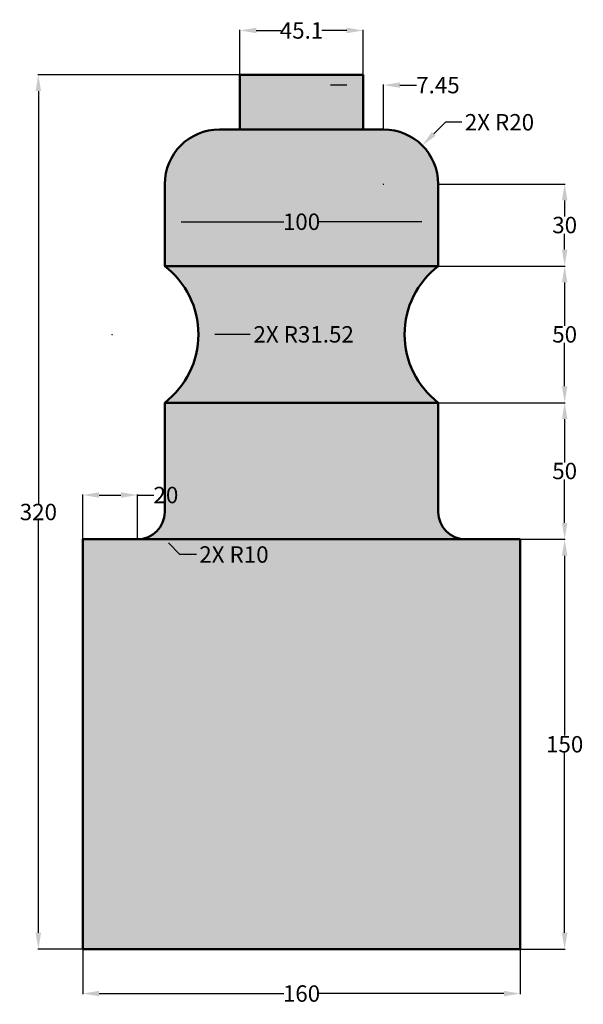
# Model space of a CAD drawing. Units: millimetres. Extents: x 528 to 734, y 162 to 523.
import ezdxf

# ---------------------------------------------------------------- set-up
doc = ezdxf.new("R2010")
doc.units = ezdxf.units.MM
doc.header["$MEASUREMENT"] = 0
doc.layers.add('M-DIMS', color=2, linetype='Continuous', lineweight=18)
doc.layers.add('M-HATC', color=18, linetype='Continuous', lineweight=18, true_color=0x000000)
doc.layers.add('M-OUTL', color=18, linetype='Continuous', lineweight=50, true_color=0x000000)
doc.styles.get("Standard").update_dxf_attribs({"font": 'arial.ttf'})
doc.dimstyles.get("Standard").update_dxf_attribs({"dimtxt": 6, "dimasz": 6, "dimexe": 0.18, "dimexo": 0.0625, "dimgap": 0.09, "dimtad": 0, "dimtih": 1, "dimtoh": 1, "dimdec": 0, "dimzin": 0, "dimdsep": 46, "dimtxsty": 'Standard', "dimcen": 0.09, "dimadec": 0, "dimazin": 0, "dimtfac": 1, "dimtdec": 0, "dimtofl": 0, "dimtmove": 0, "dimatfit": 3, "dimfxl": 1, "dimtolj": 1, "dimtzin": 0, "dimarcsym": 0})

# ---------------------------------------------------------------- blocks, each defined once
blk = doc.blocks.new('*D1')
at = {"layer": 'Defpoints', "color": 0, "transparency": 16777216}
for p in [(551.1, 182.64), (711.1, 182.64), (711.1, 166.42)]:
    blk.add_point(p, dxfattribs=at)
at = {"layer": 'M-DIMS', "color": 0, "lineweight": -2, "transparency": 16777216}
for p, q in [((551.1, 182.57), (551.1, 166.24)), ((711.1, 182.57), (711.1, 166.24)), ((557.1, 166.42), (624.67, 166.42)), ((705.1, 166.42), (637.52, 166.42))]:
    blk.add_line(p, q, dxfattribs=at)
at = {"layer": 'M-DIMS', "color": 0, "transparency": 16777216}
for points in [[(557.1, 167.42), (557.1, 165.42), (551.1, 166.42)], [(705.1, 167.42), (705.1, 165.42), (711.1, 166.42)]]:
    blk.add_solid(points, dxfattribs=at)
at = {"layer": 'M-DIMS', "color": 0, "transparency": 16777216, "insert": (631.1, 166.42), "char_height": 6, "attachment_point": 5}
blk.add_mtext('\\A1;160', dxfattribs=at)
blk = doc.blocks.new('*D2')
at = {"layer": 'Defpoints', "color": 0, "transparency": 16777216}
for p in [(653.65, 518.85), (608.55, 502.64), (653.65, 502.64)]:
    blk.add_point(p, dxfattribs=at)
at = {"layer": 'M-DIMS', "color": 0, "lineweight": -2, "transparency": 16777216}
for p, q in [((608.55, 502.7), (608.55, 519.03)), ((614.55, 518.85), (623.67, 518.85)), ((647.65, 518.85), (638.52, 518.85)), ((653.65, 502.7), (653.65, 519.03))]:
    blk.add_line(p, q, dxfattribs=at)
at = {"layer": 'M-DIMS', "color": 0, "transparency": 16777216}
for points in [[(614.55, 519.85), (614.55, 517.85), (608.55, 518.85)], [(647.65, 519.85), (647.65, 517.85), (653.65, 518.85)]]:
    blk.add_solid(points, dxfattribs=at)
at = {"layer": 'M-DIMS', "color": 0, "transparency": 16777216, "insert": (631.1, 518.85), "char_height": 6, "attachment_point": 5}
blk.add_mtext('\\A1;45.1', dxfattribs=at)
blk = doc.blocks.new('*D3')
at = {"layer": 'Defpoints', "color": 0, "transparency": 16777216}
for p in [(681.1, 448.85), (581.1, 432.64), (681.1, 432.64)]:
    blk.add_point(p, dxfattribs=at)
at = {"layer": 'M-DIMS', "color": 0, "lineweight": -2, "transparency": 16777216}
for p, q in [((581.1, 432.7), (581.1, 449.03)), ((587.1, 448.85), (624.67, 448.85)), ((675.1, 448.85), (637.52, 448.85)), ((681.1, 432.7), (681.1, 449.03))]:
    blk.add_line(p, q, dxfattribs=at)
at = {"layer": 'M-DIMS', "color": 0, "transparency": 16777216}
for points in [[(587.1, 449.85), (587.1, 447.85), (581.1, 448.85)], [(675.1, 449.85), (675.1, 447.85), (681.1, 448.85)]]:
    blk.add_solid(points, dxfattribs=at)
at = {"layer": 'M-DIMS', "color": 0, "transparency": 16777216, "insert": (631.1, 448.85), "char_height": 6, "attachment_point": 5}
blk.add_mtext('\\A1;100', dxfattribs=at)
blk = doc.blocks.new('*D4')
at = {"layer": 'Defpoints', "color": 0, "transparency": 16777216}
for p in [(571.1, 348.85), (551.1, 332.64), (571.1, 332.64)]:
    blk.add_point(p, dxfattribs=at)
at = {"layer": 'M-DIMS', "color": 0, "lineweight": -2, "transparency": 16777216}
for p, q in [((551.1, 332.7), (551.1, 349.03)), ((557.1, 348.85), (565.1, 348.85)), ((571.1, 332.7), (571.1, 349.03)), ((571.1, 348.85), (577.1, 348.85))]:
    blk.add_line(p, q, dxfattribs=at)
at = {"layer": 'M-DIMS', "color": 0, "transparency": 16777216}
for points in [[(557.1, 349.85), (557.1, 347.85), (551.1, 348.85)], [(565.1, 349.85), (565.1, 347.85), (571.1, 348.85)]]:
    blk.add_solid(points, dxfattribs=at)
at = {"layer": 'M-DIMS', "color": 0, "transparency": 16777216, "insert": (581.52, 348.85), "char_height": 6, "attachment_point": 5}
blk.add_mtext('\\A1;20', dxfattribs=at)
blk = doc.blocks.new('*D5')
at = {"layer": 'Defpoints', "color": 0, "transparency": 16777216}
for p in [(661.1, 498.85), (653.65, 482.64), (661.1, 482.64)]:
    blk.add_point(p, dxfattribs=at)
at = {"layer": 'M-DIMS', "color": 0, "lineweight": -2, "transparency": 16777216}
for p, q in [((647.65, 498.85), (641.65, 498.85)), ((653.65, 482.7), (653.65, 499.03)), ((661.1, 482.7), (661.1, 499.03)), ((667.1, 498.85), (673.1, 498.85))]:
    blk.add_line(p, q, dxfattribs=at)
at = {"layer": 'M-DIMS', "color": 0, "transparency": 16777216}
for points in [[(647.65, 499.85), (647.65, 497.85), (653.65, 498.85)], [(667.1, 499.85), (667.1, 497.85), (661.1, 498.85)]]:
    blk.add_solid(points, dxfattribs=at)
at = {"layer": 'M-DIMS', "color": 0, "transparency": 16777216, "insert": (680.98, 498.85), "char_height": 6, "attachment_point": 5}
blk.add_mtext('\\A1;7.45', dxfattribs=at)
blk = doc.blocks.new('*D6')
at = {"layer": 'Defpoints', "color": 0, "transparency": 16777216}
for p in [(534.88, 502.64), (608.55, 502.64), (551.1, 182.64)]:
    blk.add_point(p, dxfattribs=at)
at = {"layer": 'M-DIMS', "color": 0, "lineweight": -2, "transparency": 16777216}
for p, q in [((608.48, 502.64), (534.7, 502.64)), ((534.88, 496.64), (534.88, 345.79)), ((534.88, 188.64), (534.88, 339.48)), ((551.03, 182.64), (534.7, 182.64))]:
    blk.add_line(p, q, dxfattribs=at)
at = {"layer": 'M-DIMS', "color": 0, "transparency": 16777216}
for points in [[(533.88, 496.64), (535.88, 496.64), (534.88, 502.64)], [(533.88, 188.64), (535.88, 188.64), (534.88, 182.64)]]:
    blk.add_solid(points, dxfattribs=at)
at = {"layer": 'M-DIMS', "color": 0, "transparency": 16777216, "insert": (534.88, 342.64), "char_height": 6, "attachment_point": 5}
blk.add_mtext('\\A1;320', dxfattribs=at)
blk = doc.blocks.new('*D7')
at = {"layer": 'Defpoints', "color": 0, "transparency": 16777216}
for p in [(711.1, 332.64), (727.31, 332.64), (711.1, 182.64)]:
    blk.add_point(p, dxfattribs=at)
at = {"layer": 'M-DIMS', "color": 0, "lineweight": -2, "transparency": 16777216}
for p, q in [((711.16, 332.64), (727.49, 332.64)), ((727.31, 326.64), (727.31, 260.79)), ((727.31, 188.64), (727.31, 254.48)), ((711.16, 182.64), (727.49, 182.64))]:
    blk.add_line(p, q, dxfattribs=at)
at = {"layer": 'M-DIMS', "color": 0, "transparency": 16777216}
for points in [[(726.31, 326.64), (728.31, 326.64), (727.31, 332.64)], [(726.31, 188.64), (728.31, 188.64), (727.31, 182.64)]]:
    blk.add_solid(points, dxfattribs=at)
at = {"layer": 'M-DIMS', "color": 0, "transparency": 16777216, "insert": (727.31, 257.64), "char_height": 6, "attachment_point": 5}
blk.add_mtext('\\A1;150', dxfattribs=at)
blk = doc.blocks.new('*D8')
at = {"layer": 'Defpoints', "color": 0, "transparency": 16777216}
for p in [(681.1, 382.64), (727.31, 382.64), (711.1, 332.64)]:
    blk.add_point(p, dxfattribs=at)
at = {"layer": 'M-DIMS', "color": 0, "lineweight": -2, "transparency": 16777216}
for p, q in [((681.16, 382.64), (727.49, 382.64)), ((727.31, 376.64), (727.31, 360.79)), ((727.31, 338.64), (727.31, 354.48)), ((711.16, 332.64), (727.49, 332.64))]:
    blk.add_line(p, q, dxfattribs=at)
at = {"layer": 'M-DIMS', "color": 0, "transparency": 16777216}
for points in [[(726.31, 376.64), (728.31, 376.64), (727.31, 382.64)], [(726.31, 338.64), (728.31, 338.64), (727.31, 332.64)]]:
    blk.add_solid(points, dxfattribs=at)
at = {"layer": 'M-DIMS', "color": 0, "transparency": 16777216, "insert": (727.31, 357.64), "char_height": 6, "attachment_point": 5}
blk.add_mtext('\\A1;50', dxfattribs=at)
blk = doc.blocks.new('*D9')
at = {"layer": 'Defpoints', "color": 0, "transparency": 16777216}
for p in [(681.1, 432.64), (727.31, 432.64), (681.1, 382.64)]:
    blk.add_point(p, dxfattribs=at)
at = {"layer": 'M-DIMS', "color": 0, "lineweight": -2, "transparency": 16777216}
for p, q in [((681.16, 432.64), (727.49, 432.64)), ((727.31, 426.64), (727.31, 410.79)), ((727.31, 388.64), (727.31, 404.48)), ((681.16, 382.64), (727.49, 382.64))]:
    blk.add_line(p, q, dxfattribs=at)
at = {"layer": 'M-DIMS', "color": 0, "transparency": 16777216}
for points in [[(726.31, 426.64), (728.31, 426.64), (727.31, 432.64)], [(726.31, 388.64), (728.31, 388.64), (727.31, 382.64)]]:
    blk.add_solid(points, dxfattribs=at)
at = {"layer": 'M-DIMS', "color": 0, "transparency": 16777216, "insert": (727.31, 407.64), "char_height": 6, "attachment_point": 5}
blk.add_mtext('\\A1;50', dxfattribs=at)
blk = doc.blocks.new('*D10')
at = {"layer": 'Defpoints', "color": 0, "transparency": 16777216}
for p in [(681.1, 462.64), (727.31, 462.64), (681.1, 432.64)]:
    blk.add_point(p, dxfattribs=at)
at = {"layer": 'M-DIMS', "color": 0, "lineweight": -2, "transparency": 16777216}
for p, q in [((681.16, 462.64), (727.49, 462.64)), ((727.31, 456.64), (727.31, 450.79)), ((727.31, 438.64), (727.31, 444.48)), ((681.16, 432.64), (727.49, 432.64))]:
    blk.add_line(p, q, dxfattribs=at)
at = {"layer": 'M-DIMS', "color": 0, "transparency": 16777216}
for points in [[(726.31, 456.64), (728.31, 456.64), (727.31, 462.64)], [(726.31, 438.64), (728.31, 438.64), (727.31, 432.64)]]:
    blk.add_solid(points, dxfattribs=at)
at = {"layer": 'M-DIMS', "color": 0, "transparency": 16777216, "insert": (727.31, 447.64), "char_height": 6, "attachment_point": 5}
blk.add_mtext('\\A1;30', dxfattribs=at)
blk = doc.blocks.new('*D11')
at = {"layer": 'Defpoints', "color": 0, "transparency": 16777216}
for p in [(561.9, 407.64), (593.42, 407.64)]:
    blk.add_point(p, dxfattribs=at)
at = {"layer": 'M-DIMS', "color": 0, "lineweight": -2, "transparency": 16777216}
for p, q in [((561.81, 407.64), (561.99, 407.64)), ((561.9, 407.55), (561.9, 407.73)), ((612.33, 407.64), (599.42, 407.64))]:
    blk.add_line(p, q, dxfattribs=at)
at = {"layer": 'M-DIMS', "color": 0, "transparency": 16777216}
blk.add_solid([(599.42, 408.64), (599.42, 406.64), (593.42, 407.64)], dxfattribs=at)
at = {"layer": 'M-DIMS', "color": 0, "transparency": 16777216, "insert": (631.88, 407.64), "char_height": 6, "attachment_point": 5}
blk.add_mtext('\\A1;2X R31.52', dxfattribs=at)
blk = doc.blocks.new('*D12')
at = {"layer": 'Defpoints', "color": 0, "transparency": 16777216}
for p in [(675.24, 476.78), (661.1, 462.64)]:
    blk.add_point(p, dxfattribs=at)
at = {"layer": 'M-DIMS', "color": 0, "lineweight": -2, "transparency": 16777216}
for p, q in [((683.72, 485.26), (679.48, 481.02)), ((689.72, 485.26), (683.72, 485.26)), ((661.01, 462.64), (661.19, 462.64)), ((661.1, 462.55), (661.1, 462.73))]:
    blk.add_line(p, q, dxfattribs=at)
at = {"layer": 'M-DIMS', "color": 0, "transparency": 16777216}
blk.add_solid([(678.77, 481.73), (680.19, 480.31), (675.24, 476.78)], dxfattribs=at)
at = {"layer": 'M-DIMS', "color": 0, "transparency": 16777216, "insert": (703.47, 485.26), "char_height": 6, "attachment_point": 5}
blk.add_mtext('\\A1;2X R20', dxfattribs=at)
blk = doc.blocks.new('*D13')
at = {"layer": 'Defpoints', "color": 0, "transparency": 16777216}
for p in [(571.1, 342.64), (578.17, 335.57)]:
    blk.add_point(p, dxfattribs=at)
at = {"layer": 'M-DIMS', "color": 0, "lineweight": -2, "transparency": 16777216}
for p, q in [((571.01, 342.64), (571.19, 342.64)), ((571.1, 342.55), (571.1, 342.73)), ((586.65, 327.08), (582.41, 331.32)), ((592.65, 327.08), (586.65, 327.08))]:
    blk.add_line(p, q, dxfattribs=at)
at = {"layer": 'M-DIMS', "color": 0, "transparency": 16777216}
blk.add_solid([(583.12, 332.03), (581.7, 330.62), (578.17, 335.57)], dxfattribs=at)
at = {"layer": 'M-DIMS', "color": 0, "transparency": 16777216, "insert": (606.4, 327.08), "char_height": 6, "attachment_point": 5}
blk.add_mtext('\\A1;2X R10', dxfattribs=at)

msp = doc.modelspace()

# ---------------------------------------------------------------- hatches: boundary and pattern name
at = {"layer": 'M-HATC'}
h = msp.add_hatch(color=256, dxfattribs=at)
h.dxf.hatch_style = 1
h.set_gradient(color1=(188, 108, 11), color2=(254, 234, 185))
h.paths.add_polyline_path([(711.096, 332.637), (691.096, 332.637), (631.096, 332.637), (571.096, 332.637), (551.096, 332.637), (551.096, 182.637), (571.096, 182.637), (631.096, 182.637), (691.096, 182.637), (711.096, 182.637)])
h.paths.add_polyline_path([(681.096, 342.637), (681.096, 382.637), (581.096, 382.637), (581.096, 342.637, -0.4142136), (571.096, 332.637), (631.096, 332.637), (691.096, 332.637, -0.4142136)])
h.paths.add_polyline_path([(681.096, 432.637), (581.096, 432.637, -0.4930035), (581.096, 382.637), (681.096, 382.637, -0.4930035)])
h.paths.add_polyline_path([(681.096, 462.637, 0.4142136), (661.096, 482.637), (601.096, 482.637, 0.4142136), (581.096, 462.637), (581.096, 432.637), (681.096, 432.637)])
h.paths.add_polyline_path([(653.646, 502.637), (631.096, 502.637), (608.545, 502.637), (608.545, 482.637), (653.646, 482.637)])
h = msp.add_hatch(dxfattribs=at)
h.set_pattern_fill('ANSI31', color=256)
h.paths.add_polyline_path([(711.096, 332.637), (691.096, 332.637), (631.096, 332.637), (571.096, 332.637), (551.096, 332.637), (551.096, 182.637), (571.096, 182.637), (631.096, 182.637), (691.096, 182.637), (711.096, 182.637)], flags=17)
h.paths.add_polyline_path([(711.096, 332.637), (691.096, 332.637), (631.096, 332.637), (571.096, 332.637), (551.096, 332.637), (551.096, 182.637), (571.096, 182.637), (631.096, 182.637), (681.096, 182.637), (691.096, 182.637), (711.096, 182.637)], flags=17)

# ---------------------------------------------------------------- linework, layer by layer
at = {"layer": 'M-OUTL'}
for p, q in [((631.096, 502.637), (608.545, 502.637)), ((608.545, 502.637), (608.545, 482.637)), ((631.096, 502.637), (653.646, 502.637)), ((653.646, 502.637), (653.646, 482.637)), ((601.096, 482.637), (661.096, 482.637)), ((581.096, 432.637), (581.096, 462.637)), ((681.096, 462.637), (681.096, 432.637)), ((581.096, 432.637), (681.096, 432.637)), ((581.096, 342.637), (581.096, 382.637)), ((581.096, 382.637), (681.096, 382.637)), ((681.096, 342.637), (681.096, 382.637)), ((551.096, 182.637), (551.096, 332.637)), ((571.096, 332.637), (551.096, 332.637)), ((631.096, 332.637), (571.096, 332.637)), ((581.096, 332.637), (681.096, 332.637)), ((631.096, 332.637), (691.096, 332.637)), ((691.096, 332.637), (711.096, 332.637)), ((711.096, 182.637), (711.096, 332.637)), ((571.096, 182.637), (551.096, 182.637)), ((631.096, 182.637), (571.096, 182.637)), ((581.096, 182.637), (681.096, 182.637)), ((631.096, 182.637), (691.096, 182.637)), ((691.096, 182.637), (711.096, 182.637))]:
    msp.add_line(p, q, dxfattribs=at)
for centre, radius, start, end in [((601.096, 462.637), 20, 90, 180), ((661.096, 462.637), 20, 360, 90), ((561.904, 407.637), 31.517, 307.51308, 52.48692), ((700.288, 407.637), 31.517, 127.51308, 232.48692), ((571.096, 342.637), 10, 270, 0), ((691.096, 342.637), 10, 180, 270)]:
    msp.add_arc(centre, radius, start, end, dxfattribs=at)

# ---------------------------------------------------------------- dimensions: what is measured, and where the dimension line sits
at = {"layer": 'M-DIMS'}
for base, p1, p2, override, picture, middle in [((653.646, 518.852), (608.545, 502.637), (653.646, 502.637), {"dimdec": 1, "dimlfac": 1, "dimrnd": 0, "dimzin": 0, "dimdsep": 46, "dimlunit": 2}, '*D2', (631.096, 518.852)), ((661.096, 498.852), (653.646, 482.637), (661.096, 482.637), {"dimdec": 2, "dimlfac": 1, "dimrnd": 0, "dimzin": 0, "dimdsep": 46, "dimlunit": 2}, '*D5', (680.976, 498.852)), ((571.096, 348.852), (551.096, 332.637), (571.096, 332.637), {"dimdec": 0, "dimlfac": 1, "dimrnd": 0, "dimzin": 0, "dimdsep": 46, "dimlunit": 2}, '*D4', (581.524, 348.852)), ((711.096, 166.422), (551.096, 182.637), (711.096, 182.637), {"dimdec": 0, "dimlfac": 1, "dimrnd": 0, "dimzin": 0, "dimdsep": 46, "dimlunit": 2}, '*D1', (631.096, 166.422))]:
    dim = msp.add_linear_dim(base=base, p1=p1, p2=p2, dimstyle='Standard', override=override, dxfattribs=at)
    dim.commit()
    dim.dimension.update_dxf_attribs({"geometry": picture, "text_midpoint": middle})
for base, p1, p2, angle, picture, middle in [((534.881, 502.637), (551.096, 182.637), (608.545, 502.637), 90, '*D6', (534.881, 342.637)), ((727.311, 462.637), (681.096, 432.637), (681.096, 462.637), 90, '*D10', (727.311, 447.637)), ((681.096, 448.852), (581.096, 432.637), (681.096, 432.637), 0, '*D3', (631.096, 448.852)), ((727.311, 432.637), (681.096, 382.637), (681.096, 432.637), 90, '*D9', (727.311, 407.637)), ((727.311, 382.637), (711.096, 332.637), (681.096, 382.637), 90, '*D8', (727.311, 357.637)), ((727.311, 332.637), (711.096, 182.637), (711.096, 332.637), 90, '*D7', (727.311, 257.637))]:
    dim = msp.add_linear_dim(base=base, p1=p1, p2=p2, angle=angle, dimstyle='Standard', override={"dimdec": 0, "dimlfac": 1, "dimrnd": 0, "dimzin": 0, "dimdsep": 46, "dimlunit": 2}, dxfattribs=at)
    dim.commit()
    dim.dimension.update_dxf_attribs({"geometry": picture, "text_midpoint": middle})
for center, mpoint, override, picture, middle in [((661.096, 462.637), (675.238, 476.779), {"dimdec": 0, "dimlfac": 1, "dimrnd": 0, "dimzin": 0, "dimdsep": 46, "dimlunit": 2}, '*D12', (703.469, 485.264)), ((561.904, 407.637), (593.421, 407.637), {"dimdec": 2, "dimlfac": 1, "dimrnd": 0, "dimzin": 0, "dimdsep": 46, "dimlunit": 2}, '*D11', (612.331, 407.637))]:
    dim = msp.add_radius_dim(center=center, mpoint=mpoint, text='2X <>', dimstyle='Standard', override=override, dxfattribs=at)
    dim.commit()
    dim.dimension.update_dxf_attribs({"geometry": picture, "text_midpoint": middle, "dimtype": 164})
dim = msp.add_radius_dim(center=(571.096, 342.637), mpoint=(578.167, 335.566), text='2X <>', dimstyle='Standard', override={"dimdec": 0, "dimlfac": 1, "dimrnd": 0, "dimzin": 0, "dimdsep": 46, "dimlunit": 2}, dxfattribs=at)
dim.commit()
dim.dimension.update_dxf_attribs({"geometry": '*D13', "text_midpoint": (606.398, 327.081)})

doc.saveas('drawing.dxf')
